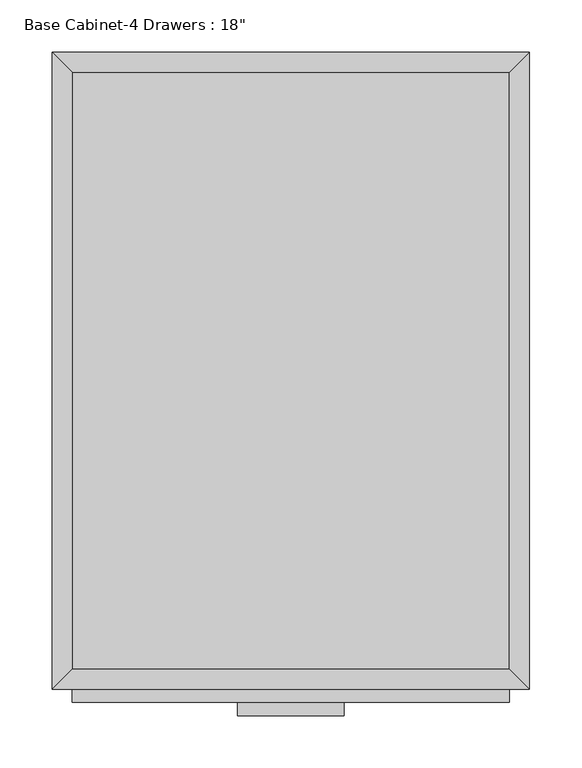
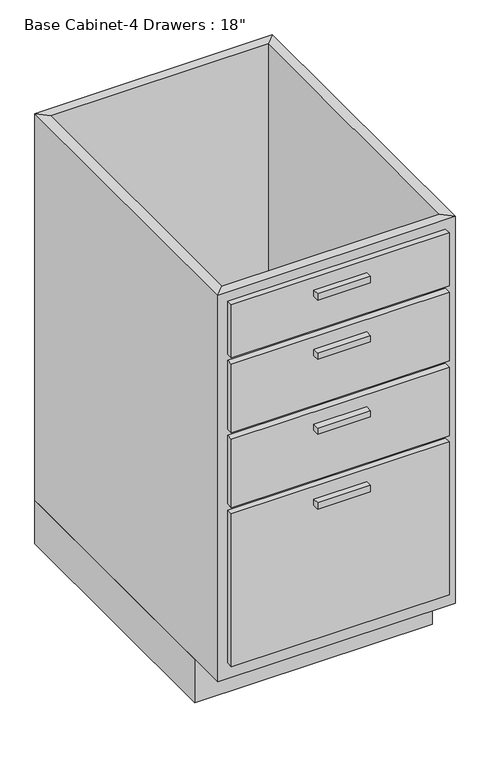
"""IFC4 building model written with IfcOpenShell, lengths in millimetres: furniture geometry."""

from ifc_helpers import new_model, si_unit, frame, origin, origin_with_axes, place, context, project, spatial, polyline, outline, extrude, faceted_brep, source, transform, mapped, element, save


def furniture_fb2da572(model_context):
    return source(origin(), model_context, "Body", "SolidModel", [
        extrude(outline(polyline([(69.5377049, -635.0), (-32.0622951, -635.0), (-32.0622951, -622.3), (69.5377049, -622.3), (69.5377049, -635.0)])), frame((0.0, 0.0, 819.15), z_axis=(0.0, 0.0, 1.0), x_axis=(1.0, 0.0, 0.0)), (0.0, 0.0, 1.0), 12.7),
        extrude(outline(polyline([(69.5377049, -635.0), (-32.0622951, -635.0), (-32.0622951, -622.3), (69.5377049, -622.3), (69.5377049, -635.0)])), frame((0.0, 0.0, 698.5), z_axis=(0.0, 0.0, 1.0), x_axis=(1.0, 0.0, 0.0)), (0.0, 0.0, 1.0), 12.7),
        extrude(outline(polyline([(69.5377049, -635.0), (-32.0622951, -635.0), (-32.0622951, -622.3), (69.5377049, -622.3), (69.5377049, -635.0)])), frame((0.0, 0.0, 546.1), z_axis=(0.0, 0.0, 1.0), x_axis=(1.0, 0.0, 0.0)), (0.0, 0.0, 1.0), 12.7),
        extrude(outline(polyline([(69.5377049, -635.0), (-32.0622951, -635.0), (-32.0622951, -622.3), (69.5377049, -622.3), (69.5377049, -635.0)])), frame((0.0, 0.0, 393.7), z_axis=(0.0, 0.0, 1.0), x_axis=(1.0, 0.0, 0.0)), (0.0, 0.0, 1.0), 12.7),
        extrude(outline(polyline([(228.2877049, -622.3), (-190.8122951, -622.3), (-190.8122951, -609.6), (228.2877049, -609.6), (228.2877049, -622.3)])), frame((0.0, 0.0, 749.3), z_axis=(0.0, 0.0, 1.0), x_axis=(1.0, 0.0, 0.0)), (0.0, 0.0, 1.0), 107.95),
        extrude(outline(polyline([(228.2877049, -622.3), (-190.8122951, -622.3), (-190.8122951, -609.6), (228.2877049, -609.6), (228.2877049, -622.3)])), frame((0.0, 0.0, 596.9), z_axis=(0.0, 0.0, 1.0), x_axis=(1.0, 0.0, 0.0)), (0.0, 0.0, 1.0), 139.7),
        extrude(outline(polyline([(228.2877049, -622.3), (-190.8122951, -622.3), (-190.8122951, -609.6), (228.2877049, -609.6), (228.2877049, -622.3)])), frame((0.0, 0.0, 444.5), z_axis=(0.0, 0.0, 1.0), x_axis=(1.0, 0.0, 0.0)), (0.0, 0.0, 1.0), 139.7),
        extrude(outline(polyline([(228.2877049, -622.3), (-190.8122951, -622.3), (-190.8122951, -609.6), (228.2877049, -609.6), (228.2877049, -622.3)])), frame((0.0, 0.0, 120.65), z_axis=(0.0, 0.0, 1.0), x_axis=(1.0, 0.0, 0.0)), (0.0, 0.0, 1.0), 311.15),
        extrude(outline(polyline([(228.2877049, -19.05), (228.2877049, -590.55), (-190.8122951, -590.55), (-190.8122951, -19.05), (228.2877049, -19.05)])), frame((0.0, 0.0, 88.9), z_axis=(0.0, 0.0, 1.0), x_axis=(1.0, 0.0, 0.0)), (0.0, 0.0, 1.0), 19.05),
        faceted_brep([(228.2877049, -590.55, 876.3), (228.2877049, -590.55, 88.9), (-190.8122951, -590.55, 88.9), (-190.8122951, -590.55, 876.3), (247.3377049, -609.6, 876.3), (-209.8622951, -609.6, 876.3), (247.3377049, -609.6, 88.9), (-209.8622951, -609.6, 88.9), (-190.8122951, -19.05, 88.9), (-190.8122951, -19.05, 876.3), (-209.8622951, 0.0, 876.3), (-209.8622951, 0.0, 88.9), (228.2877049, -19.05, 88.9), (228.2877049, -19.05, 876.3), (247.3377049, 0.0, 876.3), (247.3377049, 0.0, 88.9)], [[[0, 1, 2, 3]], [[4, 0, 3, 5]], [[6, 4, 5, 7]], [[1, 6, 7, 2]], [[3, 2, 8, 9]], [[5, 3, 9, 10]], [[7, 5, 10, 11]], [[2, 7, 11, 8]], [[9, 8, 12, 13]], [[10, 9, 13, 14]], [[11, 10, 14, 15]], [[8, 11, 15, 12]], [[13, 12, 1, 0]], [[14, 13, 0, 4]], [[15, 14, 4, 6]], [[12, 15, 6, 1]]]),
        extrude(outline(polyline([(247.3377049, 0.0), (247.3377049, -533.4), (-209.8622951, -533.4), (-209.8622951, 0.0), (247.3377049, 0.0)])), origin_with_axes(), (0.0, 0.0, 1.0), 88.9),
    ])


if __name__ == "__main__":
    model = new_model("IFC4")
    model_context = context("Model", 3, world=origin())
    ifc_project = project(units=[si_unit("LENGTHUNIT", "METRE", prefix="MILLI")], contexts=[model_context])
    site = spatial("IfcSite", under=ifc_project)
    building = spatial("IfcBuilding", under=site)
    placement = place(None, origin())
    furniture_shape = furniture_fb2da572(model_context)
    element("IfcFurniture", 1, ObjectType="Base Cabinet-4 Drawers : 18\"", at=placement, inside=building, context=model_context, shape_type="MappedRepresentation", body=[
        mapped(furniture_shape, transform((0.0, 0.0, 0.0), x_axis=(1.0, 0.0, 0.0), y_axis=(0.0, 1.0, 0.0), z_axis=(0.0, 0.0, 1.0))),
    ])
    save(model, "model.ifc")

# Revit data of these elements
# Type "Base Cabinet-4 Drawers : 18\""
#   Assembly Code = "C1030410"
#   Depth = 2' - 0"
#   Height = 2' - 10 1/2"
#   Toe Depth = 0' - 3"
#   Toe Height = 0' - 3 1/2"
#   Width = 1' - 6"
#   Cabinet Material = none
#   Door/Drawer Material = none
#   Handle Material = Cabinets - Handles
#   Default Elevation = 0
# Element 1 (IfcFurniture, "Base Cabinet-4 Drawers : 18\"")
#   Materials on its faces: "Cabinets", "Cabinets - Handles"
# Materials
#   "Cabinets - Handles": class "Metal", colour RGB 57 57 57, transparency 0
#   "Cabinets": colour RGB 249 249 249, transparency 0
